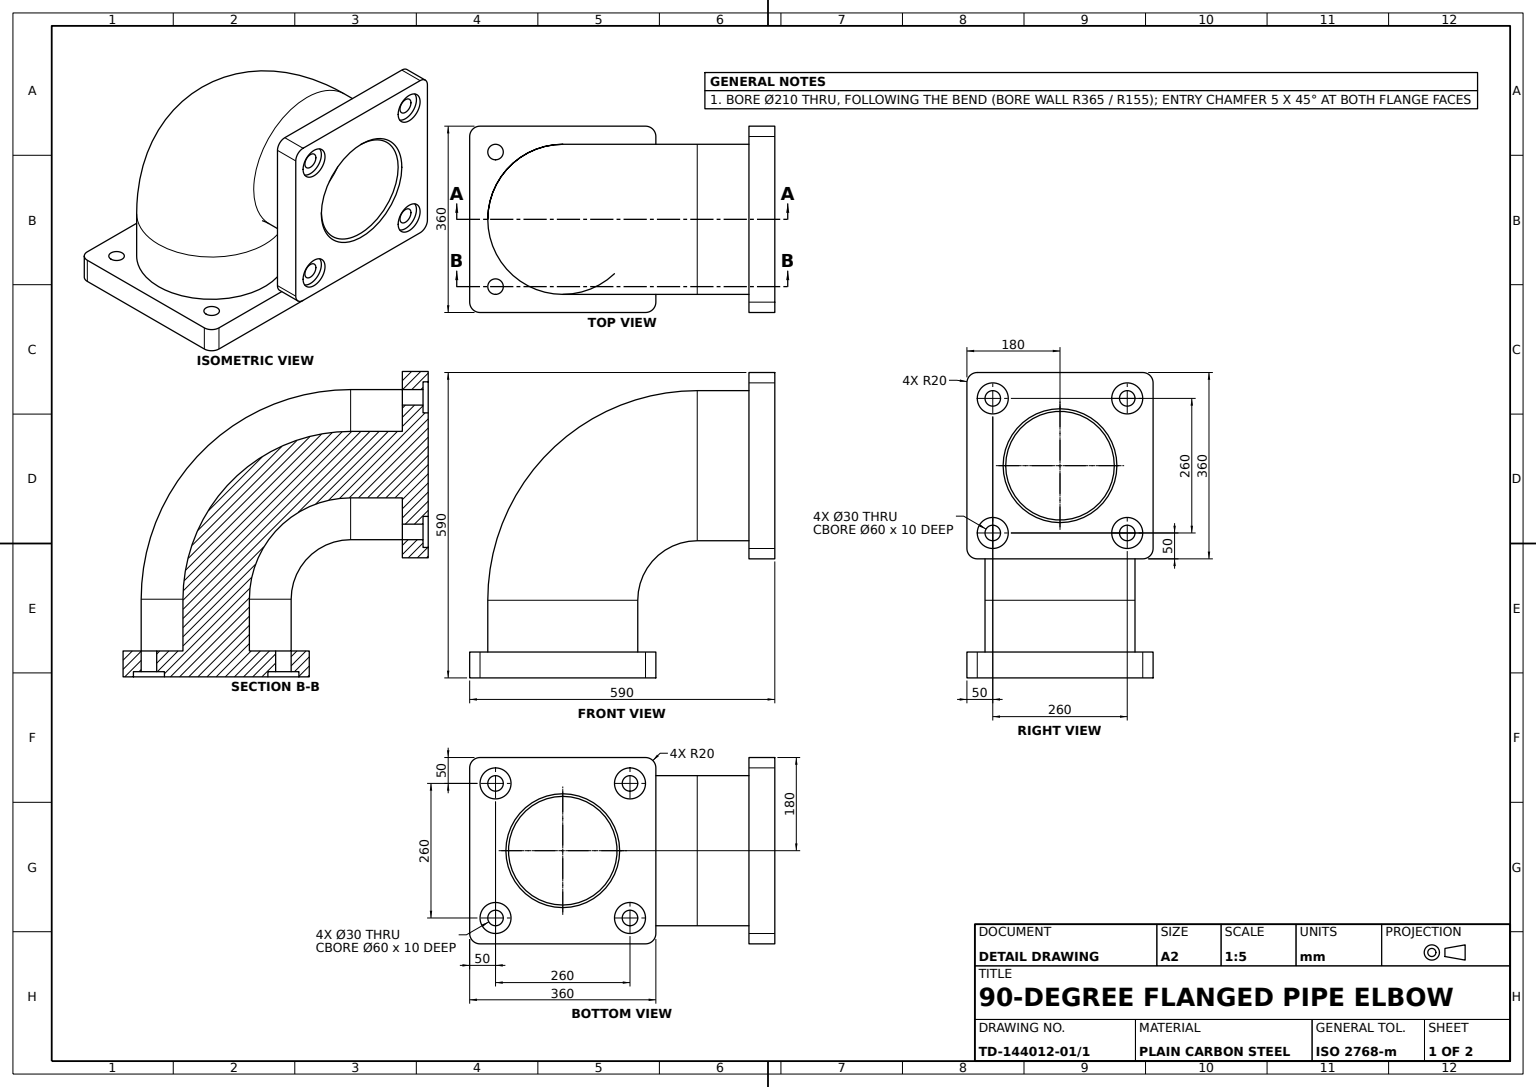
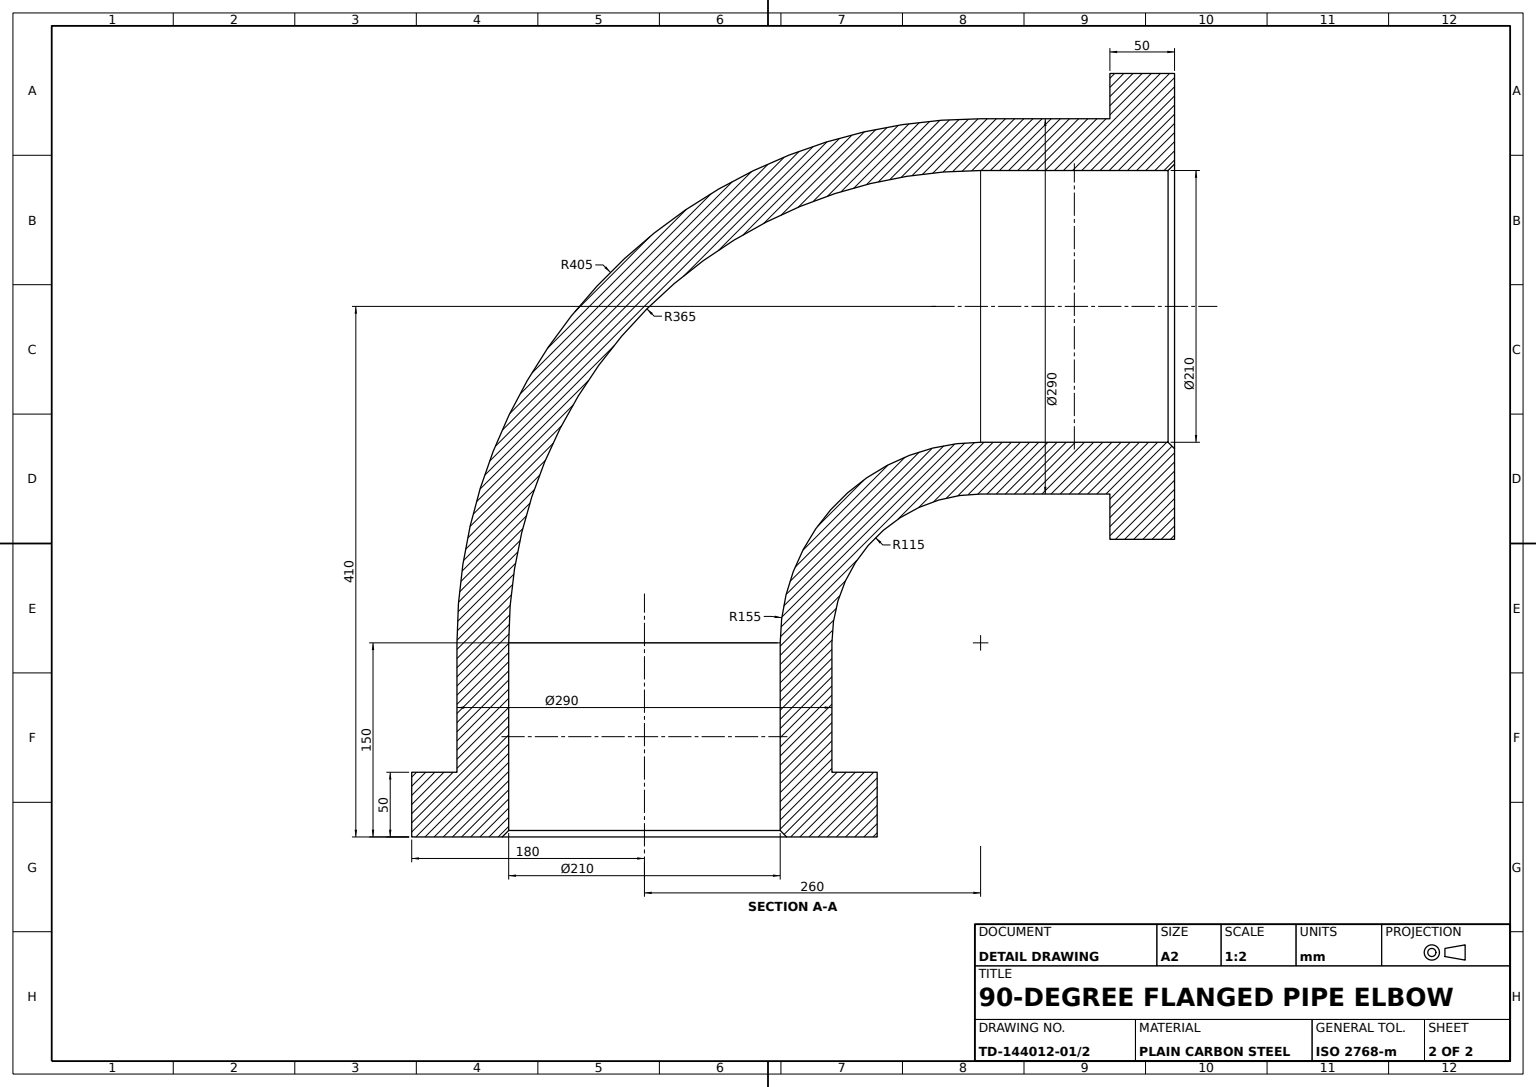
SolidWorks part; units mm, degrees
material "Plain Carbon Steel"
ref_plane "Front Plane" through (0, 0, 0) normal (0, 0, 1) x (1, 0, 0)
ref_plane "Top Plane" through (0, 0, 0) normal (0, 1, 0) x (1, 0, 0)
ref_plane "Right Plane" through (0, 0, 0) normal (1, 0, 0) x (0, 0, -1)
sketch "Elbow Path Sketch" plane through (0, 0, 0) normal (0, 0, 1) x (1, 0, 0)
  line L0 (-321.9653, 0) -> (422.5434, 0) construction
  line L1 (0, 190.4624) -> (0, -185.2601) construction
  line L2 (0, 0) -> (0, 150)
  line L3 (260, 410) -> (410, 410)
  arc A0 (0, 150) -> (260, 410) centre (260, 150) cw
  dimension "D2" = 260
  dimension "D1" = 150
  dimension "D3" = 150
ref_plane "Plane1" through (410, 0, 0) normal (1, 0, 0) x (0, 0, -1)
sketch "Elbow Section Sketch Ø210-Ø290" plane through (410, 0, 0) normal (1, 0, 0) x (0, 0, -1)
  circle A0 centre (0, 410) radius 105
  circle A1 centre (0, 410) radius 145
  dimension "D1" = 210
  dimension "D2" = 290
sweep "Elbow Body" add profiles "Elbow Section Sketch Ø210-Ø290" path "Elbow Path Sketch"
sketch "Flange A Sketch" plane through (410, 0, 0) normal (1, 0, 0) x (0, 0, -1)
  line L1 (-160, 230) -> (160, 230)
  line L2 (-180, 250) -> (-180, 570)
  line L3 (-160, 590) -> (160, 590)
  line L4 (180, 250) -> (180, 570)
  line L5 (-180, 230) -> (180, 590) construction
  line L6 (-180, 590) -> (180, 230) construction
  arc A0 (-180, 570) -> (-160, 590) centre (-160, 570) cw
  arc A1 (160, 590) -> (180, 570) centre (160, 570) cw
  arc A2 (160, 230) -> (180, 250) centre (160, 250) ccw
  arc A3 (-160, 230) -> (-180, 250) centre (-160, 250) cw
  circle A4 centre (0, 410) radius 105
  point P0 (0, 410)
  dimension "D3" = 20
  dimension "D4" = 210
  dimension "D1" = 360
  dimension "D2" = 360
extrude "Flange A 360x360x50" add sketch "Flange A Sketch" against normal blind 50
sketch "Flange B Sketch" plane through (0, 0, 0) normal (0, -1, 0) x (1, 0, 0)
  line L1 (-160, -180) -> (160, -180)
  line L2 (-180, -160) -> (-180, 160)
  line L3 (-160, 180) -> (160, 180)
  line L4 (180, -160) -> (180, 160)
  line L5 (-180, -180) -> (180, 180) construction
  line L6 (-180, 180) -> (180, -180) construction
  arc A0 (-160, -180) -> (-180, -160) centre (-160, -160) cw
  arc A1 (160, -180) -> (180, -160) centre (160, -160) ccw
  arc A2 (160, 180) -> (180, 160) centre (160, 160) cw
  arc A3 (-180, 160) -> (-160, 180) centre (-160, 160) cw
  circle A4 centre (0, 0) radius 105
  point P0 (0, 0)
  dimension "D3" = 20
  dimension "D4" = 210
  dimension "D1" = 360
  dimension "D2" = 360
extrude "Flange B 360x360x50" add sketch "Flange B Sketch" against normal blind 50
chamfer "Edge Chamfer 5x45 A" distance 5 angle 45 1 edges at (0, 0, -105)
chamfer "Edge Chamfer 5x45 B" distance 5 angle 45 1 edges at (410, 410, -105)
sketch "Flange B Bolt Holes Sketch" plane through (0, 0, 0) normal (0, -1, 0) x (1, 0, 0)
  line L0 (-293.27, 0) -> (295.2502, 0) construction
  line L1 (0, 222.6059) -> (0, -240.4398) construction
  line L2 (-180, 160) -> (-180, -160) construction
  circle A0 centre (-130, 130) radius 15
  circle A1 centre (-130, -130) radius 15
  circle A2 centre (130, -130) radius 15
  circle A3 centre (130, 130) radius 15
  dimension "D1" = 260
  dimension "D2" = 30
  dimension "D3" = 30
  dimension "D4" = 50
extrude "Flange B Bolt Holes Ø30" cut sketch "Flange B Bolt Holes Sketch" against normal blind 50
sketch "Flange B Counterbores Sketch" plane through (0, 0, 0) normal (0, -1, 0) x (1, 0, 0)
  circle A0 centre (-130, 130) radius 30
  circle A1 centre (-130, -130) radius 30
  circle A2 centre (130, -130) radius 30
  circle A3 centre (130, 130) radius 30
  dimension "D1" = 60
  dimension "D2" = 60
  dimension "D3" = 60
  dimension "D4" = 60
extrude "Flange B Counterbores Ø60x10" cut sketch "Flange B Counterbores Sketch" against normal blind 10
sketch "Flange A Bolt Holes Sketch" plane through (410, 0, 0) normal (1, 0, 0) x (0, 0, -1)
  line L0 (-180, 410) -> (225.8467, 410) construction
  line L1 (-180, 570) -> (-180, 250) construction
  line L2 (0, 663.9307) -> (0, 74.8091) construction
  circle A0 centre (-130, 540) radius 15
  circle A1 centre (-130, 280) radius 15
  circle A2 centre (130, 280) radius 15
  circle A3 centre (130, 540) radius 15
  dimension "D1" = 260
  dimension "D3" = 30
  dimension "D4" = 30
  dimension "D2" = 50
extrude "Flange A Bolt Holes Ø30" cut sketch "Flange A Bolt Holes Sketch" against normal blind 50
sketch "Flange A Counterbores Sketch" plane through (410, 0, 0) normal (1, 0, 0) x (0, 0, -1)
  circle A0 centre (-130, 540) radius 30
  circle A1 centre (130, 540) radius 30
  circle A2 centre (-130, 280) radius 30
  circle A3 centre (130, 280) radius 30
  dimension "D1" = 60
  dimension "D2" = 60
  dimension "D3" = 60
  dimension "D4" = 60
extrude "Flange A Counterbores Ø60x10" cut sketch "Flange A Counterbores Sketch" against normal blind 10
